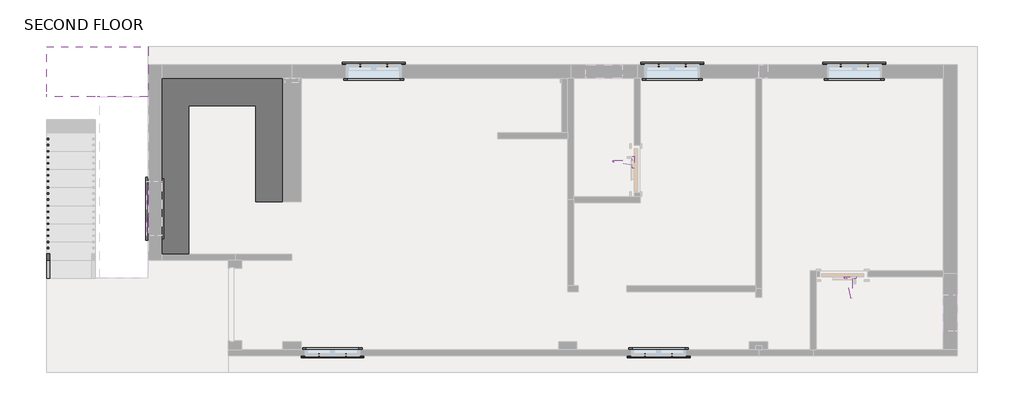
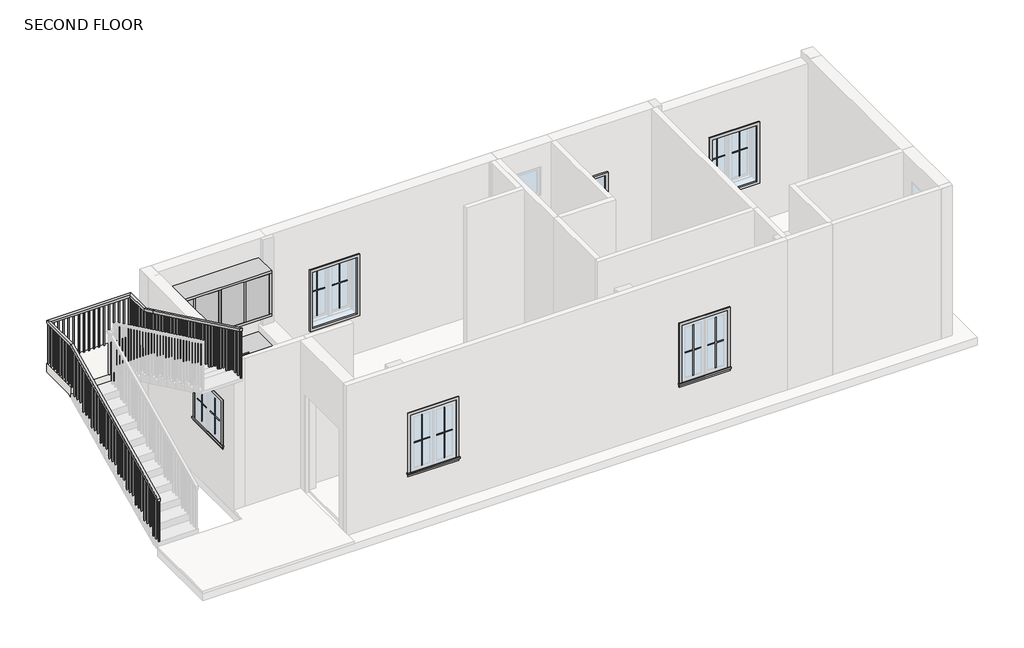
# One storey, part 3 of 3: 27 proxies, 1 railing, 1 slab.
"""IFC4 building model written with IfcOpenShell, lengths in millimetres."""

from ifc_helpers import new_model, si_unit, frame, origin, place, context, project, spatial, polyline, outline, extrude, faceted_brep, transform, mapped, element, save
from components import bel_door_closer_bel_door_closer_f210e2f3, bel_door_closer_bel_door_closer_a3520c2f, generic_models_3_generic_models_1_c5fb848b, muntin_pattern_2x2_muntin_pattern_2x2_1acec82f, muntin_pattern_2x2_muntin_pattern_2x2_43d02eee, muntin_pattern_2x2_muntin_pattern_2x2_d1c6e638, muntin_pattern_2x2_muntin_pattern_2x2_37b95fb2, trim_window_exterior_flat_with_sill_e4b28ec3, trim_window_exterior_flat_with_sill_84e24481, trim_window_interior_flat_picture_frame_39ff4276, trim_window_interior_flat_picture_frame_28d4e5dc

model = new_model("IFC4")

# Units and contexts
model_context = context("Model", 3, world=origin())
ifc_project = project(units=[si_unit("LENGTHUNIT", "METRE", prefix="MILLI")], contexts=[model_context])

# Site, building, storey
site = spatial("IfcSite", under=ifc_project)
building = spatial("IfcBuilding", under=site)
storey = spatial("IfcBuildingStorey", under=building, Name="SECOND FLOOR", Elevation=6400.8)

# Proxies
placement = place(None, origin())
bel_door_closer_bel_door_closer_shape = bel_door_closer_bel_door_closer_f210e2f3(model_context)
element("IfcBuildingElementProxy", 1, Name="BEL-Door Closer : BEL-Door Closer", ObjectType="BEL-Door Closer : BEL-Door Closer", at=placement, inside=storey, context=model_context, shape_type="MappedRepresentation", body=[
    mapped(bel_door_closer_bel_door_closer_shape, transform((6826.3533773, 1546.5642852, 8545.4957985), x_axis=(-1.0, 0.0, 0.0), y_axis=(0.0, 0.0, -1.0), z_axis=(0.0, -1.0, 0.0))),
])
bel_door_closer_bel_door_closer_2_shape = bel_door_closer_bel_door_closer_a3520c2f(model_context)
element("IfcBuildingElementProxy", 2, Name="BEL-Door Closer : BEL-Door Closer", ObjectType="BEL-Door Closer : BEL-Door Closer", at=placement, inside=storey, context=model_context, shape_type="MappedRepresentation", body=[
    mapped(bel_door_closer_bel_door_closer_2_shape, transform((3460.0408773, 3211.0767852, 8545.4957985), x_axis=(0.0, -1.0, 0.0), y_axis=(0.0, 0.0, 1.0), z_axis=(-1.0, 0.0, 0.0))),
])
generic_models_3_generic_models_1_shape = generic_models_3_generic_models_1_c5fb848b(model_context)
element("IfcBuildingElementProxy", 3, Name="Generic Models 3 : Generic Models 1", ObjectType="Generic Models 3 : Generic Models 1", at=placement, inside=storey, context=model_context, shape_type="MappedRepresentation", body=[
    mapped(generic_models_3_generic_models_1_shape, transform((0.0, 0.0, 0.0), x_axis=(1.0, 0.0, 0.0), y_axis=(0.0, 1.0, 0.0), z_axis=(0.0, 0.0, 1.0))),
])
muntin_pattern_2x2_muntin_pattern_2x2_shape = muntin_pattern_2x2_muntin_pattern_2x2_1acec82f(model_context)
element("IfcBuildingElementProxy", 4, Name="Muntin Pattern_2x2 : Muntin Pattern_2x2", ObjectType="Muntin Pattern_2x2 : Muntin Pattern_2x2", at=placement, inside=storey, context=model_context, shape_type="MappedRepresentation", body=[
    mapped(muntin_pattern_2x2_muntin_pattern_2x2_shape, transform((-1135.7716227, 5093.0392852, 7385.05), x_axis=(1.0, 0.0, 0.0), y_axis=(0.0, 1.0, 0.0), z_axis=(0.0, 0.0, 1.0))),
])
element("IfcBuildingElementProxy", 5, Name="Muntin Pattern_2x2 : Muntin Pattern_2x2", ObjectType="Muntin Pattern_2x2 : Muntin Pattern_2x2", at=placement, inside=storey, context=model_context, shape_type="MappedRepresentation", body=[
    mapped(muntin_pattern_2x2_muntin_pattern_2x2_shape, transform((3868.0283773, 5093.0392852, 7385.05), x_axis=(1.0, 0.0, 0.0), y_axis=(0.0, 1.0, 0.0), z_axis=(0.0, 0.0, 1.0))),
])
element("IfcBuildingElementProxy", 6, Name="Muntin Pattern_2x2 : Muntin Pattern_2x2", ObjectType="Muntin Pattern_2x2 : Muntin Pattern_2x2", at=placement, inside=storey, context=model_context, shape_type="MappedRepresentation", body=[
    mapped(muntin_pattern_2x2_muntin_pattern_2x2_shape, transform((6922.3783773, 5093.0392852, 7385.05), x_axis=(1.0, 0.0, 0.0), y_axis=(0.0, 1.0, 0.0), z_axis=(0.0, 0.0, 1.0))),
])
element("IfcBuildingElementProxy", 7, Name="Muntin Pattern_2x2 : Muntin Pattern_2x2", ObjectType="Muntin Pattern_2x2 : Muntin Pattern_2x2", at=placement, inside=storey, context=model_context, shape_type="MappedRepresentation", body=[
    mapped(muntin_pattern_2x2_muntin_pattern_2x2_shape, transform((4093.4533773, 235.2892852, 7385.05), x_axis=(-1.0, 0.0, 0.0), y_axis=(0.0, -1.0, 0.0), z_axis=(0.0, 0.0, 1.0))),
])
element("IfcBuildingElementProxy", 8, Name="Muntin Pattern_2x2 : Muntin Pattern_2x2", ObjectType="Muntin Pattern_2x2 : Muntin Pattern_2x2", at=placement, inside=storey, context=model_context, shape_type="MappedRepresentation", body=[
    mapped(muntin_pattern_2x2_muntin_pattern_2x2_shape, transform((-1373.8966227, 235.2892852, 7385.05), x_axis=(-1.0, 0.0, 0.0), y_axis=(0.0, -1.0, 0.0), z_axis=(0.0, 0.0, 1.0))),
])
muntin_pattern_2x2_muntin_pattern_2x2_2_shape = muntin_pattern_2x2_muntin_pattern_2x2_43d02eee(model_context)
element("IfcBuildingElementProxy", 9, Name="Muntin Pattern_2x2 : Muntin Pattern_2x2", ObjectType="Muntin Pattern_2x2 : Muntin Pattern_2x2", at=placement, inside=storey, context=model_context, shape_type="MappedRepresentation", body=[
    mapped(muntin_pattern_2x2_muntin_pattern_2x2_2_shape, transform((-681.7466227, 5093.0392852, 7385.05), x_axis=(-1.0, 0.0, 0.0), y_axis=(0.0, -1.0, 0.0), z_axis=(0.0, 0.0, 1.0))),
])
element("IfcBuildingElementProxy", 10, Name="Muntin Pattern_2x2 : Muntin Pattern_2x2", ObjectType="Muntin Pattern_2x2 : Muntin Pattern_2x2", at=placement, inside=storey, context=model_context, shape_type="MappedRepresentation", body=[
    mapped(muntin_pattern_2x2_muntin_pattern_2x2_2_shape, transform((4322.0533773, 5093.0392852, 7385.05), x_axis=(-1.0, 0.0, 0.0), y_axis=(0.0, -1.0, 0.0), z_axis=(0.0, 0.0, 1.0))),
])
element("IfcBuildingElementProxy", 11, Name="Muntin Pattern_2x2 : Muntin Pattern_2x2", ObjectType="Muntin Pattern_2x2 : Muntin Pattern_2x2", at=placement, inside=storey, context=model_context, shape_type="MappedRepresentation", body=[
    mapped(muntin_pattern_2x2_muntin_pattern_2x2_2_shape, transform((7376.4033773, 5093.0392852, 7385.05), x_axis=(-1.0, 0.0, 0.0), y_axis=(0.0, -1.0, 0.0), z_axis=(0.0, 0.0, 1.0))),
])
element("IfcBuildingElementProxy", 12, Name="Muntin Pattern_2x2 : Muntin Pattern_2x2", ObjectType="Muntin Pattern_2x2 : Muntin Pattern_2x2", at=placement, inside=storey, context=model_context, shape_type="MappedRepresentation", body=[
    mapped(muntin_pattern_2x2_muntin_pattern_2x2_2_shape, transform((3639.4283773, 235.2892852, 7385.05), x_axis=(1.0, 0.0, 0.0), y_axis=(0.0, 1.0, 0.0), z_axis=(0.0, 0.0, 1.0))),
])
element("IfcBuildingElementProxy", 13, Name="Muntin Pattern_2x2 : Muntin Pattern_2x2", ObjectType="Muntin Pattern_2x2 : Muntin Pattern_2x2", at=placement, inside=storey, context=model_context, shape_type="MappedRepresentation", body=[
    mapped(muntin_pattern_2x2_muntin_pattern_2x2_2_shape, transform((-1827.9216227, 235.2892852, 7385.05), x_axis=(1.0, 0.0, 0.0), y_axis=(0.0, 1.0, 0.0), z_axis=(0.0, 0.0, 1.0))),
])
muntin_pattern_2x2_muntin_pattern_2x2_3_shape = muntin_pattern_2x2_muntin_pattern_2x2_d1c6e638(model_context)
element("IfcBuildingElementProxy", 14, Name="Muntin Pattern_2x2 : Muntin Pattern_2x2", ObjectType="Muntin Pattern_2x2 : Muntin Pattern_2x2", at=placement, inside=storey, context=model_context, shape_type="MappedRepresentation", body=[
    mapped(muntin_pattern_2x2_muntin_pattern_2x2_3_shape, transform((-4683.8341227, 2462.5517852, 7689.85), x_axis=(0.0, 1.0, 0.0), y_axis=(-1.0, 0.0, 0.0), z_axis=(0.0, 0.0, 1.0))),
])
muntin_pattern_2x2_muntin_pattern_2x2_4_shape = muntin_pattern_2x2_muntin_pattern_2x2_37b95fb2(model_context)
element("IfcBuildingElementProxy", 15, Name="Muntin Pattern_2x2 : Muntin Pattern_2x2", ObjectType="Muntin Pattern_2x2 : Muntin Pattern_2x2", at=placement, inside=storey, context=model_context, shape_type="MappedRepresentation", body=[
    mapped(muntin_pattern_2x2_muntin_pattern_2x2_4_shape, transform((-4683.8341227, 2916.5767852, 7689.85), x_axis=(0.0, -1.0, 0.0), y_axis=(1.0, 0.0, 0.0), z_axis=(0.0, 0.0, 1.0))),
])
trim_window_exterior_flat_with_sill_shape = trim_window_exterior_flat_with_sill_e4b28ec3(model_context)
element("IfcBuildingElementProxy", 16, Name="Trim-Window-Exterior-Flat : with Sill", ObjectType="Trim-Window-Exterior-Flat : with Sill", at=placement, inside=storey, context=model_context, shape_type="MappedRepresentation", body=[
    mapped(trim_window_exterior_flat_with_sill_shape, transform((-908.7591227, 5102.5642852, 8534.4), x_axis=(-1.0, 0.0, 0.0), y_axis=(0.0, 0.0, 1.0), z_axis=(0.0, 1.0, 0.0))),
])
element("IfcBuildingElementProxy", 17, Name="Trim-Window-Exterior-Flat : with Sill", ObjectType="Trim-Window-Exterior-Flat : with Sill", at=placement, inside=storey, context=model_context, shape_type="MappedRepresentation", body=[
    mapped(trim_window_exterior_flat_with_sill_shape, transform((4095.0408773, 5102.5642852, 8534.4), x_axis=(-1.0, 0.0, 0.0), y_axis=(0.0, 0.0, 1.0), z_axis=(0.0, 1.0, 0.0))),
])
element("IfcBuildingElementProxy", 18, Name="Trim-Window-Exterior-Flat : with Sill", ObjectType="Trim-Window-Exterior-Flat : with Sill", at=placement, inside=storey, context=model_context, shape_type="MappedRepresentation", body=[
    mapped(trim_window_exterior_flat_with_sill_shape, transform((7149.3908773, 5102.5642852, 8534.4), x_axis=(-1.0, 0.0, 0.0), y_axis=(0.0, 0.0, 1.0), z_axis=(0.0, 1.0, 0.0))),
])
element("IfcBuildingElementProxy", 19, Name="Trim-Window-Exterior-Flat : with Sill", ObjectType="Trim-Window-Exterior-Flat : with Sill", at=placement, inside=storey, context=model_context, shape_type="MappedRepresentation", body=[
    mapped(trim_window_exterior_flat_with_sill_shape, transform((3866.4408773, 225.7642852, 8534.4), x_axis=(1.0, 0.0, 0.0), y_axis=(0.0, 0.0, 1.0), z_axis=(0.0, -1.0, 0.0))),
])
element("IfcBuildingElementProxy", 20, Name="Trim-Window-Exterior-Flat : with Sill", ObjectType="Trim-Window-Exterior-Flat : with Sill", at=placement, inside=storey, context=model_context, shape_type="MappedRepresentation", body=[
    mapped(trim_window_exterior_flat_with_sill_shape, transform((-1600.9091227, 225.7642852, 8534.4), x_axis=(1.0, 0.0, 0.0), y_axis=(0.0, 0.0, 1.0), z_axis=(0.0, -1.0, 0.0))),
])
trim_window_exterior_flat_with_sill_2_shape = trim_window_exterior_flat_with_sill_84e24481(model_context)
element("IfcBuildingElementProxy", 21, Name="Trim-Window-Exterior-Flat : with Sill", ObjectType="Trim-Window-Exterior-Flat : with Sill", at=placement, inside=storey, context=model_context, shape_type="MappedRepresentation", body=[
    mapped(trim_window_exterior_flat_with_sill_2_shape, transform((-4693.3591227, 2689.5642852, 8534.4), x_axis=(0.0, -1.0, 0.0), y_axis=(0.0, 0.0, 1.0), z_axis=(-1.0, 0.0, 0.0))),
])
trim_window_interior_flat_picture_frame_shape = trim_window_interior_flat_picture_frame_39ff4276(model_context)
element("IfcBuildingElementProxy", 22, Name="Trim-Window-Interior-Flat : Picture Frame", ObjectType="Trim-Window-Interior-Flat : Picture Frame", at=placement, inside=storey, context=model_context, shape_type="MappedRepresentation", body=[
    mapped(trim_window_interior_flat_picture_frame_shape, transform((-908.7591227, 4873.9642852, 8534.4), x_axis=(1.0, 0.0, 0.0), y_axis=(0.0, 0.0, 1.0), z_axis=(0.0, -1.0, 0.0))),
])
element("IfcBuildingElementProxy", 23, Name="Trim-Window-Interior-Flat : Picture Frame", ObjectType="Trim-Window-Interior-Flat : Picture Frame", at=placement, inside=storey, context=model_context, shape_type="MappedRepresentation", body=[
    mapped(trim_window_interior_flat_picture_frame_shape, transform((4095.0408773, 4873.9642852, 8534.4), x_axis=(1.0, 0.0, 0.0), y_axis=(0.0, 0.0, 1.0), z_axis=(0.0, -1.0, 0.0))),
])
element("IfcBuildingElementProxy", 24, Name="Trim-Window-Interior-Flat : Picture Frame", ObjectType="Trim-Window-Interior-Flat : Picture Frame", at=placement, inside=storey, context=model_context, shape_type="MappedRepresentation", body=[
    mapped(trim_window_interior_flat_picture_frame_shape, transform((7149.3908773, 4873.9642852, 8534.4), x_axis=(1.0, 0.0, 0.0), y_axis=(0.0, 0.0, 1.0), z_axis=(0.0, -1.0, 0.0))),
])
element("IfcBuildingElementProxy", 25, Name="Trim-Window-Interior-Flat : Picture Frame", ObjectType="Trim-Window-Interior-Flat : Picture Frame", at=placement, inside=storey, context=model_context, shape_type="MappedRepresentation", body=[
    mapped(trim_window_interior_flat_picture_frame_shape, transform((3866.4408773, 327.3642852, 8534.4), x_axis=(-1.0, 0.0, 0.0), y_axis=(0.0, 0.0, 1.0), z_axis=(0.0, 1.0, 0.0))),
])
element("IfcBuildingElementProxy", 26, Name="Trim-Window-Interior-Flat : Picture Frame", ObjectType="Trim-Window-Interior-Flat : Picture Frame", at=placement, inside=storey, context=model_context, shape_type="MappedRepresentation", body=[
    mapped(trim_window_interior_flat_picture_frame_shape, transform((-1600.9091227, 327.3642852, 8534.4), x_axis=(-1.0, 0.0, 0.0), y_axis=(0.0, 0.0, 1.0), z_axis=(0.0, 1.0, 0.0))),
])
trim_window_interior_flat_picture_frame_2_shape = trim_window_interior_flat_picture_frame_28d4e5dc(model_context)
element("IfcBuildingElementProxy", 27, Name="Trim-Window-Interior-Flat : Picture Frame", ObjectType="Trim-Window-Interior-Flat : Picture Frame", at=placement, inside=storey, context=model_context, shape_type="MappedRepresentation", body=[
    mapped(trim_window_interior_flat_picture_frame_2_shape, transform((-4464.7591227, 2689.5642852, 8534.4), x_axis=(0.0, 1.0, 0.0), y_axis=(0.0, 0.0, 1.0), z_axis=(1.0, 0.0, 0.0))),
])

# Railing
element("IfcRailing", 28, ObjectType="Handrail - Rectangular", at=placement, inside=storey, context=model_context, shape_type="SolidModel", body=[
    faceted_brep([(-6395.1591227, 1521.1642852, 7460.6727273), (-6395.1591227, 1521.1642852, 7404.3834559), (-6344.3591227, 1521.1642852, 7404.3834559), (-6344.3591227, 1521.1642852, 7460.6727273), (-6395.1591227, 4569.1642852, 8915.4), (-6395.1591227, 4580.6656156, 8864.6), (-6344.3591227, 4580.6656156, 8864.6), (-6344.3591227, 4569.1642852, 8915.4), (-6395.1591227, 5407.3642852, 8915.4), (-6395.1591227, 5407.3642852, 8864.6), (-6344.3591227, 5356.5642852, 8864.6), (-6344.3591227, 5356.5642852, 8915.4), (-4693.3591227, 5407.3642852, 8915.4), (-4693.3591227, 5407.3642852, 8864.6), (-4744.1591227, 5356.5642852, 8864.6), (-4744.1591227, 5356.5642852, 8915.4), (-4693.3591227, 4873.9642852, 8915.4), (-4693.3591227, 4862.4629548, 8864.6), (-4744.1591227, 4862.4629548, 8864.6), (-4744.1591227, 4873.9642852, 8915.4), (-4693.3591227, 4569.1642852, 9060.8727273), (-4693.3591227, 4547.2832222, 9015.0266906), (-4744.1591227, 4547.2832222, 9015.0266906), (-4744.1591227, 4569.1642852, 9060.8727273), (-4693.3591227, 1521.1642852, 10515.6), (-4744.1591227, 1521.1642852, 10515.6), (-4744.1591227, 1521.1642852, 10459.3107287), (-4693.3591227, 1521.1642852, 10459.3107287)], [[[0, 1, 2, 3]], [[1, 0, 4, 5]], [[2, 1, 5, 6]], [[3, 2, 6, 7]], [[0, 3, 7, 4]], [[5, 4, 8, 9]], [[6, 5, 9, 10]], [[7, 6, 10, 11]], [[4, 7, 11, 8]], [[9, 8, 12, 13]], [[10, 9, 13, 14]], [[11, 10, 14, 15]], [[8, 11, 15, 12]], [[13, 12, 16, 17]], [[14, 13, 17, 18]], [[15, 14, 18, 19]], [[12, 15, 19, 16]], [[17, 16, 20, 21]], [[18, 17, 21, 22]], [[19, 18, 22, 23]], [[16, 19, 23, 20]], [[24, 25, 26, 27]], [[21, 20, 24, 27]], [[22, 21, 27, 26]], [[23, 22, 26, 25]], [[20, 23, 25, 24]]]),
    extrude(outline(polyline([(1632.2892852, 10406.2737969), (1632.2892852, 9455.7272727), (1613.2392852, 9455.7272727), (1613.2392852, 10415.3658423), (1632.2892852, 10406.2737969)])), frame((-4728.2841227, 0.0, 0.0), z_axis=(1.0, 0.0, 0.0), x_axis=(0.0, 1.0, 0.0)), (0.0, 0.0, 1.0), 19.05),
    extrude(outline(polyline([(1733.8892852, 10357.7828878), (1733.8892852, 9455.7272727), (1714.8392852, 9455.7272727), (1714.8392852, 10366.8749332), (1733.8892852, 10357.7828878)])), frame((-4728.2841227, 0.0, 0.0), z_axis=(1.0, 0.0, 0.0), x_axis=(0.0, 1.0, 0.0)), (0.0, 0.0, 1.0), 19.05),
    extrude(outline(polyline([(1835.4892852, 10309.2919787), (1835.4892852, 9455.7272727), (1816.4392852, 9455.7272727), (1816.4392852, 10318.3840241), (1835.4892852, 10309.2919787)])), frame((-4728.2841227, 0.0, 0.0), z_axis=(1.0, 0.0, 0.0), x_axis=(0.0, 1.0, 0.0)), (0.0, 0.0, 1.0), 19.05),
    extrude(outline(polyline([(1937.0892852, 10260.8010696), (1937.0892852, 9310.2545455), (1918.0392852, 9310.2545455), (1918.0392852, 10269.893115), (1937.0892852, 10260.8010696)])), frame((-4728.2841227, 0.0, 0.0), z_axis=(1.0, 0.0, 0.0), x_axis=(0.0, 1.0, 0.0)), (0.0, 0.0, 1.0), 19.05),
    extrude(outline(polyline([(2038.6892852, 10212.3101605), (2038.6892852, 9310.2545455), (2019.6392852, 9310.2545455), (2019.6392852, 10221.4022059), (2038.6892852, 10212.3101605)])), frame((-4728.2841227, 0.0, 0.0), z_axis=(1.0, 0.0, 0.0), x_axis=(0.0, 1.0, 0.0)), (0.0, 0.0, 1.0), 19.05),
    extrude(outline(polyline([(2140.2892852, 10163.8192514), (2140.2892852, 9310.2545455), (2121.2392852, 9310.2545455), (2121.2392852, 10172.9112969), (2140.2892852, 10163.8192514)])), frame((-4728.2841227, 0.0, 0.0), z_axis=(1.0, 0.0, 0.0), x_axis=(0.0, 1.0, 0.0)), (0.0, 0.0, 1.0), 19.05),
    extrude(outline(polyline([(2241.8892852, 10115.3283423), (2241.8892852, 9164.7818182), (2222.8392852, 9164.7818182), (2222.8392852, 10124.4203878), (2241.8892852, 10115.3283423)])), frame((-4728.2841227, 0.0, 0.0), z_axis=(1.0, 0.0, 0.0), x_axis=(0.0, 1.0, 0.0)), (0.0, 0.0, 1.0), 19.05),
    extrude(outline(polyline([(2343.4892852, 10066.8374332), (2343.4892852, 9164.7818182), (2324.4392852, 9164.7818182), (2324.4392852, 10075.9294787), (2343.4892852, 10066.8374332)])), frame((-4728.2841227, 0.0, 0.0), z_axis=(1.0, 0.0, 0.0), x_axis=(0.0, 1.0, 0.0)), (0.0, 0.0, 1.0), 19.05),
    extrude(outline(polyline([(2445.0892852, 10018.3465241), (2445.0892852, 9164.7818182), (2426.0392852, 9164.7818182), (2426.0392852, 10027.4385696), (2445.0892852, 10018.3465241)])), frame((-4728.2841227, 0.0, 0.0), z_axis=(1.0, 0.0, 0.0), x_axis=(0.0, 1.0, 0.0)), (0.0, 0.0, 1.0), 19.05),
    extrude(outline(polyline([(2546.6892852, 9969.855615), (2546.6892852, 9019.3090909), (2527.6392852, 9019.3090909), (2527.6392852, 9978.9476605), (2546.6892852, 9969.855615)])), frame((-4728.2841227, 0.0, 0.0), z_axis=(1.0, 0.0, 0.0), x_axis=(0.0, 1.0, 0.0)), (0.0, 0.0, 1.0), 19.05),
    extrude(outline(polyline([(2648.2892852, 9921.3647059), (2648.2892852, 9019.3090909), (2629.2392852, 9019.3090909), (2629.2392852, 9930.4567514), (2648.2892852, 9921.3647059)])), frame((-4728.2841227, 0.0, 0.0), z_axis=(1.0, 0.0, 0.0), x_axis=(0.0, 1.0, 0.0)), (0.0, 0.0, 1.0), 19.05),
    extrude(outline(polyline([(2749.8892852, 9872.8737969), (2749.8892852, 9019.3090909), (2730.8392852, 9019.3090909), (2730.8392852, 9881.9658423), (2749.8892852, 9872.8737969)])), frame((-4728.2841227, 0.0, 0.0), z_axis=(1.0, 0.0, 0.0), x_axis=(0.0, 1.0, 0.0)), (0.0, 0.0, 1.0), 19.05),
    extrude(outline(polyline([(2851.4892852, 9824.3828878), (2851.4892852, 8873.8363636), (2832.4392852, 8873.8363636), (2832.4392852, 9833.4749332), (2851.4892852, 9824.3828878)])), frame((-4728.2841227, 0.0, 0.0), z_axis=(1.0, 0.0, 0.0), x_axis=(0.0, 1.0, 0.0)), (0.0, 0.0, 1.0), 19.05),
    extrude(outline(polyline([(2953.0892852, 9775.8919787), (2953.0892852, 8873.8363636), (2934.0392852, 8873.8363636), (2934.0392852, 9784.9840241), (2953.0892852, 9775.8919787)])), frame((-4728.2841227, 0.0, 0.0), z_axis=(1.0, 0.0, 0.0), x_axis=(0.0, 1.0, 0.0)), (0.0, 0.0, 1.0), 19.05),
    extrude(outline(polyline([(3054.6892852, 9727.4010696), (3054.6892852, 8873.8363636), (3035.6392852, 8873.8363636), (3035.6392852, 9736.493115), (3054.6892852, 9727.4010696)])), frame((-4728.2841227, 0.0, 0.0), z_axis=(1.0, 0.0, 0.0), x_axis=(0.0, 1.0, 0.0)), (0.0, 0.0, 1.0), 19.05),
    extrude(outline(polyline([(3156.2892852, 9678.9101605), (3156.2892852, 8728.3636364), (3137.2392852, 8728.3636364), (3137.2392852, 9688.0022059), (3156.2892852, 9678.9101605)])), frame((-4728.2841227, 0.0, 0.0), z_axis=(1.0, 0.0, 0.0), x_axis=(0.0, 1.0, 0.0)), (0.0, 0.0, 1.0), 19.05),
    extrude(outline(polyline([(3257.8892852, 9630.4192514), (3257.8892852, 8728.3636364), (3238.8392852, 8728.3636364), (3238.8392852, 9639.5112969), (3257.8892852, 9630.4192514)])), frame((-4728.2841227, 0.0, 0.0), z_axis=(1.0, 0.0, 0.0), x_axis=(0.0, 1.0, 0.0)), (0.0, 0.0, 1.0), 19.05),
    extrude(outline(polyline([(3359.4892852, 9581.9283423), (3359.4892852, 8728.3636364), (3340.4392852, 8728.3636364), (3340.4392852, 9591.0203878), (3359.4892852, 9581.9283423)])), frame((-4728.2841227, 0.0, 0.0), z_axis=(1.0, 0.0, 0.0), x_axis=(0.0, 1.0, 0.0)), (0.0, 0.0, 1.0), 19.05),
    extrude(outline(polyline([(3461.0892852, 9533.4374332), (3461.0892852, 8582.8909091), (3442.0392852, 8582.8909091), (3442.0392852, 9542.5294787), (3461.0892852, 9533.4374332)])), frame((-4728.2841227, 0.0, 0.0), z_axis=(1.0, 0.0, 0.0), x_axis=(0.0, 1.0, 0.0)), (0.0, 0.0, 1.0), 19.05),
    extrude(outline(polyline([(3562.6892852, 9484.9465241), (3562.6892852, 8582.8909091), (3543.6392852, 8582.8909091), (3543.6392852, 9494.0385696), (3562.6892852, 9484.9465241)])), frame((-4728.2841227, 0.0, 0.0), z_axis=(1.0, 0.0, 0.0), x_axis=(0.0, 1.0, 0.0)), (0.0, 0.0, 1.0), 19.05),
    extrude(outline(polyline([(3664.2892852, 9436.455615), (3664.2892852, 8582.8909091), (3645.2392852, 8582.8909091), (3645.2392852, 9445.5476605), (3664.2892852, 9436.455615)])), frame((-4728.2841227, 0.0, 0.0), z_axis=(1.0, 0.0, 0.0), x_axis=(0.0, 1.0, 0.0)), (0.0, 0.0, 1.0), 19.05),
    extrude(outline(polyline([(3765.8892852, 9387.9647059), (3765.8892852, 8437.4181818), (3746.8392852, 8437.4181818), (3746.8392852, 9397.0567514), (3765.8892852, 9387.9647059)])), frame((-4728.2841227, 0.0, 0.0), z_axis=(1.0, 0.0, 0.0), x_axis=(0.0, 1.0, 0.0)), (0.0, 0.0, 1.0), 19.05),
    extrude(outline(polyline([(3867.4892852, 9339.4737969), (3867.4892852, 8437.4181818), (3848.4392852, 8437.4181818), (3848.4392852, 9348.5658423), (3867.4892852, 9339.4737969)])), frame((-4728.2841227, 0.0, 0.0), z_axis=(1.0, 0.0, 0.0), x_axis=(0.0, 1.0, 0.0)), (0.0, 0.0, 1.0), 19.05),
    extrude(outline(polyline([(3969.0892852, 9290.9828878), (3969.0892852, 8437.4181818), (3950.0392852, 8437.4181818), (3950.0392852, 9300.0749332), (3969.0892852, 9290.9828878)])), frame((-4728.2841227, 0.0, 0.0), z_axis=(1.0, 0.0, 0.0), x_axis=(0.0, 1.0, 0.0)), (0.0, 0.0, 1.0), 19.05),
    extrude(outline(polyline([(4070.6892852, 9242.4919787), (4070.6892852, 8291.9454545), (4051.6392852, 8291.9454545), (4051.6392852, 9251.5840241), (4070.6892852, 9242.4919787)])), frame((-4728.2841227, 0.0, 0.0), z_axis=(1.0, 0.0, 0.0), x_axis=(0.0, 1.0, 0.0)), (0.0, 0.0, 1.0), 19.05),
    extrude(outline(polyline([(4172.2892852, 9194.0010696), (4172.2892852, 8291.9454545), (4153.2392852, 8291.9454545), (4153.2392852, 9203.093115), (4172.2892852, 9194.0010696)])), frame((-4728.2841227, 0.0, 0.0), z_axis=(1.0, 0.0, 0.0), x_axis=(0.0, 1.0, 0.0)), (0.0, 0.0, 1.0), 19.05),
    extrude(outline(polyline([(4273.8892852, 9145.5101605), (4273.8892852, 8291.9454545), (4254.8392852, 8291.9454545), (4254.8392852, 9154.6022059), (4273.8892852, 9145.5101605)])), frame((-4728.2841227, 0.0, 0.0), z_axis=(1.0, 0.0, 0.0), x_axis=(0.0, 1.0, 0.0)), (0.0, 0.0, 1.0), 19.05),
    extrude(outline(polyline([(4375.4892852, 9097.0192514), (4375.4892852, 8146.4727273), (4356.4392852, 8146.4727273), (4356.4392852, 9106.1112969), (4375.4892852, 9097.0192514)])), frame((-4728.2841227, 0.0, 0.0), z_axis=(1.0, 0.0, 0.0), x_axis=(0.0, 1.0, 0.0)), (0.0, 0.0, 1.0), 19.05),
    extrude(outline(polyline([(4477.0892852, 9048.5283423), (4477.0892852, 8146.4727273), (4458.0392852, 8146.4727273), (4458.0392852, 9057.6203878), (4477.0892852, 9048.5283423)])), frame((-4728.2841227, 0.0, 0.0), z_axis=(1.0, 0.0, 0.0), x_axis=(0.0, 1.0, 0.0)), (0.0, 0.0, 1.0), 19.05),
    extrude(outline(polyline([(4680.2892852, 8951.5465241), (4680.2892852, 8001.0), (4661.2392852, 8001.0), (4661.2392852, 8960.6385696), (4680.2892852, 8951.5465241)])), frame((-4728.2841227, 0.0, 0.0), z_axis=(1.0, 0.0, 0.0), x_axis=(0.0, 1.0, 0.0)), (0.0, 0.0, 1.0), 19.05),
    extrude(outline(polyline([(4781.8892852, 8903.055615), (4781.8892852, 8001.0), (4762.8392852, 8001.0), (4762.8392852, 8912.1476605), (4781.8892852, 8903.055615)])), frame((-4728.2841227, 0.0, 0.0), z_axis=(1.0, 0.0, 0.0), x_axis=(0.0, 1.0, 0.0)), (0.0, 0.0, 1.0), 19.05),
    extrude(outline(polyline([(-4709.2341227, 4883.4892852), (-4709.2341227, 4864.4392852), (-4728.2841227, 4864.4392852), (-4728.2841227, 4883.4892852), (-4709.2341227, 4883.4892852)])), frame((0.0, 0.0, 8001.0), z_axis=(0.0, 0.0, 1.0), x_axis=(1.0, 0.0, 0.0)), (0.0, 0.0, 1.0), 863.6),
    extrude(outline(polyline([(-4709.2341227, 4985.0892852), (-4709.2341227, 4966.0392852), (-4728.2841227, 4966.0392852), (-4728.2841227, 4985.0892852), (-4709.2341227, 4985.0892852)])), frame((0.0, 0.0, 8001.0), z_axis=(0.0, 0.0, 1.0), x_axis=(1.0, 0.0, 0.0)), (0.0, 0.0, 1.0), 863.6),
    extrude(outline(polyline([(-4709.2341227, 5086.6892852), (-4709.2341227, 5067.6392852), (-4728.2841227, 5067.6392852), (-4728.2841227, 5086.6892852), (-4709.2341227, 5086.6892852)])), frame((0.0, 0.0, 8001.0), z_axis=(0.0, 0.0, 1.0), x_axis=(1.0, 0.0, 0.0)), (0.0, 0.0, 1.0), 863.6),
    extrude(outline(polyline([(-4709.2341227, 5188.2892852), (-4709.2341227, 5169.2392852), (-4728.2841227, 5169.2392852), (-4728.2841227, 5188.2892852), (-4709.2341227, 5188.2892852)])), frame((0.0, 0.0, 8001.0), z_axis=(0.0, 0.0, 1.0), x_axis=(1.0, 0.0, 0.0)), (0.0, 0.0, 1.0), 863.6),
    extrude(outline(polyline([(-4709.2341227, 5289.8892852), (-4709.2341227, 5270.8392852), (-4728.2841227, 5270.8392852), (-4728.2841227, 5289.8892852), (-4709.2341227, 5289.8892852)])), frame((0.0, 0.0, 8001.0), z_axis=(0.0, 0.0, 1.0), x_axis=(1.0, 0.0, 0.0)), (0.0, 0.0, 1.0), 863.6),
    extrude(outline(polyline([(-4753.6841227, 5391.4892852), (-4734.6341227, 5391.4892852), (-4734.6341227, 5372.4392852), (-4753.6841227, 5372.4392852), (-4753.6841227, 5391.4892852)])), frame((0.0, 0.0, 8001.0), z_axis=(0.0, 0.0, 1.0), x_axis=(1.0, 0.0, 0.0)), (0.0, 0.0, 1.0), 863.6),
    extrude(outline(polyline([(-4855.2841227, 5391.4892852), (-4836.2341227, 5391.4892852), (-4836.2341227, 5372.4392852), (-4855.2841227, 5372.4392852), (-4855.2841227, 5391.4892852)])), frame((0.0, 0.0, 8001.0), z_axis=(0.0, 0.0, 1.0), x_axis=(1.0, 0.0, 0.0)), (0.0, 0.0, 1.0), 863.6),
    extrude(outline(polyline([(-4956.8841227, 5391.4892852), (-4937.8341227, 5391.4892852), (-4937.8341227, 5372.4392852), (-4956.8841227, 5372.4392852), (-4956.8841227, 5391.4892852)])), frame((0.0, 0.0, 8001.0), z_axis=(0.0, 0.0, 1.0), x_axis=(1.0, 0.0, 0.0)), (0.0, 0.0, 1.0), 863.6),
    extrude(outline(polyline([(-5058.4841227, 5391.4892852), (-5039.4341227, 5391.4892852), (-5039.4341227, 5372.4392852), (-5058.4841227, 5372.4392852), (-5058.4841227, 5391.4892852)])), frame((0.0, 0.0, 8001.0), z_axis=(0.0, 0.0, 1.0), x_axis=(1.0, 0.0, 0.0)), (0.0, 0.0, 1.0), 863.6),
    extrude(outline(polyline([(-5160.0841227, 5391.4892852), (-5141.0341227, 5391.4892852), (-5141.0341227, 5372.4392852), (-5160.0841227, 5372.4392852), (-5160.0841227, 5391.4892852)])), frame((0.0, 0.0, 8001.0), z_axis=(0.0, 0.0, 1.0), x_axis=(1.0, 0.0, 0.0)), (0.0, 0.0, 1.0), 863.6),
    extrude(outline(polyline([(-5261.6841227, 5391.4892852), (-5242.6341227, 5391.4892852), (-5242.6341227, 5372.4392852), (-5261.6841227, 5372.4392852), (-5261.6841227, 5391.4892852)])), frame((0.0, 0.0, 8001.0), z_axis=(0.0, 0.0, 1.0), x_axis=(1.0, 0.0, 0.0)), (0.0, 0.0, 1.0), 863.6),
    extrude(outline(polyline([(-5363.2841227, 5391.4892852), (-5344.2341227, 5391.4892852), (-5344.2341227, 5372.4392852), (-5363.2841227, 5372.4392852), (-5363.2841227, 5391.4892852)])), frame((0.0, 0.0, 8001.0), z_axis=(0.0, 0.0, 1.0), x_axis=(1.0, 0.0, 0.0)), (0.0, 0.0, 1.0), 863.6),
    extrude(outline(polyline([(-5464.8841227, 5391.4892852), (-5445.8341227, 5391.4892852), (-5445.8341227, 5372.4392852), (-5464.8841227, 5372.4392852), (-5464.8841227, 5391.4892852)])), frame((0.0, 0.0, 8001.0), z_axis=(0.0, 0.0, 1.0), x_axis=(1.0, 0.0, 0.0)), (0.0, 0.0, 1.0), 863.6),
    extrude(outline(polyline([(-5566.4841227, 5391.4892852), (-5547.4341227, 5391.4892852), (-5547.4341227, 5372.4392852), (-5566.4841227, 5372.4392852), (-5566.4841227, 5391.4892852)])), frame((0.0, 0.0, 8001.0), z_axis=(0.0, 0.0, 1.0), x_axis=(1.0, 0.0, 0.0)), (0.0, 0.0, 1.0), 863.6),
    extrude(outline(polyline([(-5668.0841227, 5391.4892852), (-5649.0341227, 5391.4892852), (-5649.0341227, 5372.4392852), (-5668.0841227, 5372.4392852), (-5668.0841227, 5391.4892852)])), frame((0.0, 0.0, 8001.0), z_axis=(0.0, 0.0, 1.0), x_axis=(1.0, 0.0, 0.0)), (0.0, 0.0, 1.0), 863.6),
    extrude(outline(polyline([(-5769.6841227, 5391.4892852), (-5750.6341227, 5391.4892852), (-5750.6341227, 5372.4392852), (-5769.6841227, 5372.4392852), (-5769.6841227, 5391.4892852)])), frame((0.0, 0.0, 8001.0), z_axis=(0.0, 0.0, 1.0), x_axis=(1.0, 0.0, 0.0)), (0.0, 0.0, 1.0), 863.6),
    extrude(outline(polyline([(-5871.2841227, 5391.4892852), (-5852.2341227, 5391.4892852), (-5852.2341227, 5372.4392852), (-5871.2841227, 5372.4392852), (-5871.2841227, 5391.4892852)])), frame((0.0, 0.0, 8001.0), z_axis=(0.0, 0.0, 1.0), x_axis=(1.0, 0.0, 0.0)), (0.0, 0.0, 1.0), 863.6),
    extrude(outline(polyline([(-5972.8841227, 5391.4892852), (-5953.8341227, 5391.4892852), (-5953.8341227, 5372.4392852), (-5972.8841227, 5372.4392852), (-5972.8841227, 5391.4892852)])), frame((0.0, 0.0, 8001.0), z_axis=(0.0, 0.0, 1.0), x_axis=(1.0, 0.0, 0.0)), (0.0, 0.0, 1.0), 863.6),
    extrude(outline(polyline([(-6074.4841227, 5391.4892852), (-6055.4341227, 5391.4892852), (-6055.4341227, 5372.4392852), (-6074.4841227, 5372.4392852), (-6074.4841227, 5391.4892852)])), frame((0.0, 0.0, 8001.0), z_axis=(0.0, 0.0, 1.0), x_axis=(1.0, 0.0, 0.0)), (0.0, 0.0, 1.0), 863.6),
    extrude(outline(polyline([(-6176.0841227, 5391.4892852), (-6157.0341227, 5391.4892852), (-6157.0341227, 5372.4392852), (-6176.0841227, 5372.4392852), (-6176.0841227, 5391.4892852)])), frame((0.0, 0.0, 8001.0), z_axis=(0.0, 0.0, 1.0), x_axis=(1.0, 0.0, 0.0)), (0.0, 0.0, 1.0), 863.6),
    extrude(outline(polyline([(-6277.6841227, 5391.4892852), (-6258.6341227, 5391.4892852), (-6258.6341227, 5372.4392852), (-6277.6841227, 5372.4392852), (-6277.6841227, 5391.4892852)])), frame((0.0, 0.0, 8001.0), z_axis=(0.0, 0.0, 1.0), x_axis=(1.0, 0.0, 0.0)), (0.0, 0.0, 1.0), 863.6),
    extrude(outline(polyline([(-6379.2841227, 5270.8392852), (-6379.2841227, 5289.8892852), (-6360.2341227, 5289.8892852), (-6360.2341227, 5270.8392852), (-6379.2841227, 5270.8392852)])), frame((0.0, 0.0, 8001.0), z_axis=(0.0, 0.0, 1.0), x_axis=(1.0, 0.0, 0.0)), (0.0, 0.0, 1.0), 863.6),
    extrude(outline(polyline([(-6379.2841227, 5169.2392852), (-6379.2841227, 5188.2892852), (-6360.2341227, 5188.2892852), (-6360.2341227, 5169.2392852), (-6379.2841227, 5169.2392852)])), frame((0.0, 0.0, 8001.0), z_axis=(0.0, 0.0, 1.0), x_axis=(1.0, 0.0, 0.0)), (0.0, 0.0, 1.0), 863.6),
    extrude(outline(polyline([(-6379.2841227, 5067.6392852), (-6379.2841227, 5086.6892852), (-6360.2341227, 5086.6892852), (-6360.2341227, 5067.6392852), (-6379.2841227, 5067.6392852)])), frame((0.0, 0.0, 8001.0), z_axis=(0.0, 0.0, 1.0), x_axis=(1.0, 0.0, 0.0)), (0.0, 0.0, 1.0), 863.6),
    extrude(outline(polyline([(-6379.2841227, 4966.0392852), (-6379.2841227, 4985.0892852), (-6360.2341227, 4985.0892852), (-6360.2341227, 4966.0392852), (-6379.2841227, 4966.0392852)])), frame((0.0, 0.0, 8001.0), z_axis=(0.0, 0.0, 1.0), x_axis=(1.0, 0.0, 0.0)), (0.0, 0.0, 1.0), 863.6),
    extrude(outline(polyline([(-6379.2841227, 4864.4392852), (-6379.2841227, 4883.4892852), (-6360.2341227, 4883.4892852), (-6360.2341227, 4864.4392852), (-6379.2841227, 4864.4392852)])), frame((0.0, 0.0, 8001.0), z_axis=(0.0, 0.0, 1.0), x_axis=(1.0, 0.0, 0.0)), (0.0, 0.0, 1.0), 863.6),
    extrude(outline(polyline([(-6379.2841227, 4762.8392852), (-6379.2841227, 4781.8892852), (-6360.2341227, 4781.8892852), (-6360.2341227, 4762.8392852), (-6379.2841227, 4762.8392852)])), frame((0.0, 0.0, 8001.0), z_axis=(0.0, 0.0, 1.0), x_axis=(1.0, 0.0, 0.0)), (0.0, 0.0, 1.0), 863.6),
    extrude(outline(polyline([(-6379.2841227, 4661.2392852), (-6379.2841227, 4680.2892852), (-6360.2341227, 4680.2892852), (-6360.2341227, 4661.2392852), (-6379.2841227, 4661.2392852)])), frame((0.0, 0.0, 8001.0), z_axis=(0.0, 0.0, 1.0), x_axis=(1.0, 0.0, 0.0)), (0.0, 0.0, 1.0), 863.6),
    extrude(outline(polyline([(4477.0892852, 8815.1658423), (4477.0892852, 7855.5272727), (4458.0392852, 7855.5272727), (4458.0392852, 8806.0737969), (4477.0892852, 8815.1658423)])), frame((-6379.2841227, 0.0, 0.0), z_axis=(1.0, 0.0, 0.0), x_axis=(0.0, 1.0, 0.0)), (0.0, 0.0, 1.0), 19.05),
    extrude(outline(polyline([(4375.4892852, 8766.6749332), (4375.4892852, 7855.5272727), (4356.4392852, 7855.5272727), (4356.4392852, 8757.5828878), (4375.4892852, 8766.6749332)])), frame((-6379.2841227, 0.0, 0.0), z_axis=(1.0, 0.0, 0.0), x_axis=(0.0, 1.0, 0.0)), (0.0, 0.0, 1.0), 19.05),
    extrude(outline(polyline([(4273.8892852, 8718.1840241), (4273.8892852, 7855.5272727), (4254.8392852, 7855.5272727), (4254.8392852, 8709.0919787), (4273.8892852, 8718.1840241)])), frame((-6379.2841227, 0.0, 0.0), z_axis=(1.0, 0.0, 0.0), x_axis=(0.0, 1.0, 0.0)), (0.0, 0.0, 1.0), 19.05),
    extrude(outline(polyline([(4172.2892852, 8669.693115), (4172.2892852, 7710.0545455), (4153.2392852, 7710.0545455), (4153.2392852, 8660.6010696), (4172.2892852, 8669.693115)])), frame((-6379.2841227, 0.0, 0.0), z_axis=(1.0, 0.0, 0.0), x_axis=(0.0, 1.0, 0.0)), (0.0, 0.0, 1.0), 19.05),
    extrude(outline(polyline([(4070.6892852, 8621.2022059), (4070.6892852, 7710.0545455), (4051.6392852, 7710.0545455), (4051.6392852, 8612.1101605), (4070.6892852, 8621.2022059)])), frame((-6379.2841227, 0.0, 0.0), z_axis=(1.0, 0.0, 0.0), x_axis=(0.0, 1.0, 0.0)), (0.0, 0.0, 1.0), 19.05),
    extrude(outline(polyline([(3969.0892852, 8572.7112969), (3969.0892852, 7710.0545455), (3950.0392852, 7710.0545455), (3950.0392852, 8563.6192514), (3969.0892852, 8572.7112969)])), frame((-6379.2841227, 0.0, 0.0), z_axis=(1.0, 0.0, 0.0), x_axis=(0.0, 1.0, 0.0)), (0.0, 0.0, 1.0), 19.05),
    extrude(outline(polyline([(3867.4892852, 8524.2203878), (3867.4892852, 7564.5818182), (3848.4392852, 7564.5818182), (3848.4392852, 8515.1283423), (3867.4892852, 8524.2203878)])), frame((-6379.2841227, 0.0, 0.0), z_axis=(1.0, 0.0, 0.0), x_axis=(0.0, 1.0, 0.0)), (0.0, 0.0, 1.0), 19.05),
    extrude(outline(polyline([(3765.8892852, 8475.7294787), (3765.8892852, 7564.5818182), (3746.8392852, 7564.5818182), (3746.8392852, 8466.6374332), (3765.8892852, 8475.7294787)])), frame((-6379.2841227, 0.0, 0.0), z_axis=(1.0, 0.0, 0.0), x_axis=(0.0, 1.0, 0.0)), (0.0, 0.0, 1.0), 19.05),
    extrude(outline(polyline([(3664.2892852, 8427.2385696), (3664.2892852, 7564.5818182), (3645.2392852, 7564.5818182), (3645.2392852, 8418.1465241), (3664.2892852, 8427.2385696)])), frame((-6379.2841227, 0.0, 0.0), z_axis=(1.0, 0.0, 0.0), x_axis=(0.0, 1.0, 0.0)), (0.0, 0.0, 1.0), 19.05),
    extrude(outline(polyline([(3562.6892852, 8378.7476605), (3562.6892852, 7419.1090909), (3543.6392852, 7419.1090909), (3543.6392852, 8369.655615), (3562.6892852, 8378.7476605)])), frame((-6379.2841227, 0.0, 0.0), z_axis=(1.0, 0.0, 0.0), x_axis=(0.0, 1.0, 0.0)), (0.0, 0.0, 1.0), 19.05),
    extrude(outline(polyline([(3461.0892852, 8330.2567514), (3461.0892852, 7419.1090909), (3442.0392852, 7419.1090909), (3442.0392852, 8321.1647059), (3461.0892852, 8330.2567514)])), frame((-6379.2841227, 0.0, 0.0), z_axis=(1.0, 0.0, 0.0), x_axis=(0.0, 1.0, 0.0)), (0.0, 0.0, 1.0), 19.05),
    extrude(outline(polyline([(3359.4892852, 8281.7658423), (3359.4892852, 7419.1090909), (3340.4392852, 7419.1090909), (3340.4392852, 8272.6737969), (3359.4892852, 8281.7658423)])), frame((-6379.2841227, 0.0, 0.0), z_axis=(1.0, 0.0, 0.0), x_axis=(0.0, 1.0, 0.0)), (0.0, 0.0, 1.0), 19.05),
    extrude(outline(polyline([(3257.8892852, 8233.2749332), (3257.8892852, 7273.6363636), (3238.8392852, 7273.6363636), (3238.8392852, 8224.1828878), (3257.8892852, 8233.2749332)])), frame((-6379.2841227, 0.0, 0.0), z_axis=(1.0, 0.0, 0.0), x_axis=(0.0, 1.0, 0.0)), (0.0, 0.0, 1.0), 19.05),
    extrude(outline(polyline([(3156.2892852, 8184.7840241), (3156.2892852, 7273.6363636), (3137.2392852, 7273.6363636), (3137.2392852, 8175.6919787), (3156.2892852, 8184.7840241)])), frame((-6379.2841227, 0.0, 0.0), z_axis=(1.0, 0.0, 0.0), x_axis=(0.0, 1.0, 0.0)), (0.0, 0.0, 1.0), 19.05),
    extrude(outline(polyline([(3054.6892852, 8136.293115), (3054.6892852, 7273.6363636), (3035.6392852, 7273.6363636), (3035.6392852, 8127.2010696), (3054.6892852, 8136.293115)])), frame((-6379.2841227, 0.0, 0.0), z_axis=(1.0, 0.0, 0.0), x_axis=(0.0, 1.0, 0.0)), (0.0, 0.0, 1.0), 19.05),
    extrude(outline(polyline([(2953.0892852, 8087.8022059), (2953.0892852, 7128.1636364), (2934.0392852, 7128.1636364), (2934.0392852, 8078.7101605), (2953.0892852, 8087.8022059)])), frame((-6379.2841227, 0.0, 0.0), z_axis=(1.0, 0.0, 0.0), x_axis=(0.0, 1.0, 0.0)), (0.0, 0.0, 1.0), 19.05),
    extrude(outline(polyline([(2851.4892852, 8039.3112969), (2851.4892852, 7128.1636364), (2832.4392852, 7128.1636364), (2832.4392852, 8030.2192514), (2851.4892852, 8039.3112969)])), frame((-6379.2841227, 0.0, 0.0), z_axis=(1.0, 0.0, 0.0), x_axis=(0.0, 1.0, 0.0)), (0.0, 0.0, 1.0), 19.05),
    extrude(outline(polyline([(2749.8892852, 7990.8203878), (2749.8892852, 7128.1636364), (2730.8392852, 7128.1636364), (2730.8392852, 7981.7283423), (2749.8892852, 7990.8203878)])), frame((-6379.2841227, 0.0, 0.0), z_axis=(1.0, 0.0, 0.0), x_axis=(0.0, 1.0, 0.0)), (0.0, 0.0, 1.0), 19.05),
    extrude(outline(polyline([(2648.2892852, 7942.3294787), (2648.2892852, 6982.6909091), (2629.2392852, 6982.6909091), (2629.2392852, 7933.2374332), (2648.2892852, 7942.3294787)])), frame((-6379.2841227, 0.0, 0.0), z_axis=(1.0, 0.0, 0.0), x_axis=(0.0, 1.0, 0.0)), (0.0, 0.0, 1.0), 19.05),
    extrude(outline(polyline([(2546.6892852, 7893.8385696), (2546.6892852, 6982.6909091), (2527.6392852, 6982.6909091), (2527.6392852, 7884.7465241), (2546.6892852, 7893.8385696)])), frame((-6379.2841227, 0.0, 0.0), z_axis=(1.0, 0.0, 0.0), x_axis=(0.0, 1.0, 0.0)), (0.0, 0.0, 1.0), 19.05),
    extrude(outline(polyline([(2445.0892852, 7845.3476605), (2445.0892852, 6982.6909091), (2426.0392852, 6982.6909091), (2426.0392852, 7836.255615), (2445.0892852, 7845.3476605)])), frame((-6379.2841227, 0.0, 0.0), z_axis=(1.0, 0.0, 0.0), x_axis=(0.0, 1.0, 0.0)), (0.0, 0.0, 1.0), 19.05),
    extrude(outline(polyline([(2343.4892852, 7796.8567514), (2343.4892852, 6837.2181818), (2324.4392852, 6837.2181818), (2324.4392852, 7787.7647059), (2343.4892852, 7796.8567514)])), frame((-6379.2841227, 0.0, 0.0), z_axis=(1.0, 0.0, 0.0), x_axis=(0.0, 1.0, 0.0)), (0.0, 0.0, 1.0), 19.05),
    extrude(outline(polyline([(2241.8892852, 7748.3658423), (2241.8892852, 6837.2181818), (2222.8392852, 6837.2181818), (2222.8392852, 7739.2737969), (2241.8892852, 7748.3658423)])), frame((-6379.2841227, 0.0, 0.0), z_axis=(1.0, 0.0, 0.0), x_axis=(0.0, 1.0, 0.0)), (0.0, 0.0, 1.0), 19.05),
    extrude(outline(polyline([(2140.2892852, 7699.8749332), (2140.2892852, 6837.2181818), (2121.2392852, 6837.2181818), (2121.2392852, 7690.7828878), (2140.2892852, 7699.8749332)])), frame((-6379.2841227, 0.0, 0.0), z_axis=(1.0, 0.0, 0.0), x_axis=(0.0, 1.0, 0.0)), (0.0, 0.0, 1.0), 19.05),
    extrude(outline(polyline([(2038.6892852, 7651.3840241), (2038.6892852, 6691.7454545), (2019.6392852, 6691.7454545), (2019.6392852, 7642.2919787), (2038.6892852, 7651.3840241)])), frame((-6379.2841227, 0.0, 0.0), z_axis=(1.0, 0.0, 0.0), x_axis=(0.0, 1.0, 0.0)), (0.0, 0.0, 1.0), 19.05),
    extrude(outline(polyline([(1937.0892852, 7602.893115), (1937.0892852, 6691.7454545), (1918.0392852, 6691.7454545), (1918.0392852, 7593.8010696), (1937.0892852, 7602.893115)])), frame((-6379.2841227, 0.0, 0.0), z_axis=(1.0, 0.0, 0.0), x_axis=(0.0, 1.0, 0.0)), (0.0, 0.0, 1.0), 19.05),
    extrude(outline(polyline([(1835.4892852, 7554.4022059), (1835.4892852, 6691.7454545), (1816.4392852, 6691.7454545), (1816.4392852, 7545.3101605), (1835.4892852, 7554.4022059)])), frame((-6379.2841227, 0.0, 0.0), z_axis=(1.0, 0.0, 0.0), x_axis=(0.0, 1.0, 0.0)), (0.0, 0.0, 1.0), 19.05),
    extrude(outline(polyline([(1733.8892852, 7505.9112969), (1733.8892852, 6546.2727273), (1714.8392852, 6546.2727273), (1714.8392852, 7496.8192514), (1733.8892852, 7505.9112969)])), frame((-6379.2841227, 0.0, 0.0), z_axis=(1.0, 0.0, 0.0), x_axis=(0.0, 1.0, 0.0)), (0.0, 0.0, 1.0), 19.05),
    extrude(outline(polyline([(1632.2892852, 7457.4203878), (1632.2892852, 6546.2727273), (1613.2392852, 6546.2727273), (1613.2392852, 7448.3283423), (1632.2892852, 7457.4203878)])), frame((-6379.2841227, 0.0, 0.0), z_axis=(1.0, 0.0, 0.0), x_axis=(0.0, 1.0, 0.0)), (0.0, 0.0, 1.0), 19.05),
    extrude(outline(polyline([(4578.6892852, 9000.0374332), (4578.6892852, 8001.0), (4559.6392852, 8001.0), (4559.6392852, 9009.1294787), (4578.6892852, 9000.0374332)])), frame((-4728.2841227, 0.0, 0.0), z_axis=(1.0, 0.0, 0.0), x_axis=(0.0, 1.0, 0.0)), (0.0, 0.0, 1.0), 19.05),
    extrude(outline(polyline([(-4728.2841227, 5391.4892852), (-4709.2341227, 5391.4892852), (-4709.2341227, 5372.4392852), (-4728.2841227, 5372.4392852), (-4728.2841227, 5391.4892852)])), frame((0.0, 0.0, 8001.0), z_axis=(0.0, 0.0, 1.0), x_axis=(1.0, 0.0, 0.0)), (0.0, 0.0, 1.0), 863.6),
    extrude(outline(polyline([(-6379.2841227, 5372.4392852), (-6379.2841227, 5391.4892852), (-6360.2341227, 5391.4892852), (-6360.2341227, 5372.4392852), (-6379.2841227, 5372.4392852)])), frame((0.0, 0.0, 8001.0), z_axis=(0.0, 0.0, 1.0), x_axis=(1.0, 0.0, 0.0)), (0.0, 0.0, 1.0), 863.6),
    extrude(outline(polyline([(4578.6892852, 8863.6567514), (4578.6892852, 8001.0), (4559.6392852, 8001.0), (4559.6392852, 8854.5647059), (4578.6892852, 8863.6567514)])), frame((-6379.2841227, 0.0, 0.0), z_axis=(1.0, 0.0, 0.0), x_axis=(0.0, 1.0, 0.0)), (0.0, 0.0, 1.0), 19.05),
    extrude(outline(polyline([(1540.2142852, 10450.2186832), (1540.2142852, 9455.7272727), (1521.1642852, 9455.7272727), (1521.1642852, 10459.3107287), (1540.2142852, 10450.2186832)])), frame((-4728.2841227, 0.0, 0.0), z_axis=(1.0, 0.0, 0.0), x_axis=(0.0, 1.0, 0.0)), (0.0, 0.0, 1.0), 19.05),
    extrude(outline(polyline([(1540.2142852, 7413.4755014), (1540.2142852, 6546.2727273), (1521.1642852, 6546.2727273), (1521.1642852, 7404.3834559), (1540.2142852, 7413.4755014)])), frame((-6379.2841227, 0.0, 0.0), z_axis=(1.0, 0.0, 0.0), x_axis=(0.0, 1.0, 0.0)), (0.0, 0.0, 1.0), 19.05),
])

# Slab
element("IfcSlab", 29, ObjectType="7\" Thickness", at=placement, inside=storey, context=model_context, shape_type="Brep", body=[
    faceted_brep([(-6395.1591227, 4569.1642852, 8001.0), (-5582.3591227, 4569.1642852, 8001.0), (-5506.1591227, 4569.1642852, 8001.0), (-4693.3591227, 4569.1642852, 8001.0), (-4693.3591227, 4794.2733365, 8001.0), (-4693.3591227, 5407.3642852, 8001.0), (-6395.1591227, 5407.3642852, 8001.0), (-6395.1591227, 4648.8552339, 8001.0), (-6395.1591227, 4569.1642852, 7855.5272727), (-6395.1591227, 4569.1642852, 7785.1656836), (-5582.3591227, 4569.1642852, 7785.1656836), (-5582.3591227, 4569.1642852, 7823.2), (-5506.1591227, 4569.1642852, 7823.2), (-5506.1591227, 4569.1642852, 7930.6384108), (-4693.3591227, 4569.1642852, 7930.6384108), (-4693.3591227, 4794.2733365, 7823.2), (-4693.3591227, 5407.3642852, 7823.2), (-6395.1591227, 5407.3642852, 7823.2), (-6395.1591227, 4648.8552339, 7823.2), (-5506.1591227, 4794.2733365, 7823.2), (-5582.3591227, 4648.8552339, 7823.2)], [[[0, 1, 2, 3, 4, 5, 6, 7]], [[1, 0, 8, 9, 10, 11]], [[2, 1, 11, 12, 13]], [[3, 2, 13, 14]], [[3, 14, 15, 16, 5, 4]], [[6, 5, 16, 17]], [[9, 8, 0, 7, 6, 17, 18]], [[19, 12, 11, 20, 18, 17, 16, 15]], [[12, 19, 13]], [[18, 20, 10, 9]], [[20, 11, 10]], [[19, 15, 14, 13]]]),
])

save(model, "model.ifc")

# Revit data of these elements
# Type "BEL-Door Closer : BEL-Door Closer"
#   URL = "http://us.allegion.com/brands/falcon/Pages/default.aspx"
#   Standards Conformance = "as Specified"
#   Specification = ""
#   SpecWizard = ""
#   Send Message = "http://arcat.com/users.pl?action=UserEmail&company=Falcon+Lock&coid=32420&rep=114&fax=&mf="
#   Screw Pack Type = "as Specified"
#   Sales Information = "http://us.allegion.com/irst/Pages/contact_us.aspx"
#   Revision = "R1_02-2014"
#   Product Properties = ""
#   Product Data = "http://www.arcat.com/arcatcos/cos32/arc32420.html"
#   Model = "As Specified"
#   Manufacturer Website = "http://us.allegion.com/brands/falcon/Pages/default.aspx"
#   Manufacturer Phone = ""
#   Manufacturer Fax = ""
#   Manufacturer = "Falcon"
#   Keynote = "08710"
#   Installation-Fabrication = ""
#   Installation Phase = ""
#   Green Building-LEED = ""
#   Function Type = "as Specified"
#   Door Type = "as Specified"
#   Description = "Falcon Closer as Specified"
#   Copyright = "©Arcat Inc."
#   Construction Details = ""
#   Assembly Code = "C1020410"
#   originlocate [instance default] = 0' - 0"
#   locatearm [instance default] = 0' - 0 1/2"
#   Unit Width = 0' - 7.87402"
#   Unit Height = 0' - 3.14961"
#   Unit Depth = 0' - 1.1811"
#   Plate Thickness = 0' - 0 1/4"
#   Offset from Edge of Frame_Closer Arm [instance default] = 0' - 7"
#   Offset from Edge of Door_Closer Case [instance default] = 0' - 3 15/16"
#   Offset for Plate [instance default] = 0' - 0"
#   Reveal Between Door and Frame_Right [instance default] = 0' - 0 1/4"
#   Reveal Between Door and Frame_Left [instance default] = 0' - 0 1/4"
#   Door Leaf Width [instance default] = 3' - 0"
#   Door Leaf Top Reveal [instance default] = 0' - 0 1/4"
#   Door Leaf Thickness [instance default] = 0' - 0"
#   Closer Case Side Offset = 0' - 3 15/16"
#   Closer Arm Offset = 0' - 7"
#   Arm Width = 1' - 2"
#   Arm Height = 0' - 1 5/8"
#   Arm Extension [instance default] = 0' - 0"
#   Arm Depth = 1' - 2"
#   ActualArm Height [instance default] = 0' - 1 7/8"
#   ActualArm Depth [instance default] = 1' - 2"
#   Warranty Duration (Years) = 0
#   RH Hinge [instance default] = no
#   Maintenance Schedule (Months) = 0
#   LH Hinge [instance default] = yes
#   Include Mounting Plate [instance default] = no
#   Expected Lifespan (Years) = 0
#   Closer on Door Surface = yes
#   Closer on Door Frame = no
#   Arm Below Closer = no
#   Arm Above Closer = yes
#   Cover Material [instance default] = Metal - IR - Satin Chrome
#   Arm Type = element 418778
#   Arm Material [instance default] = Metal - IR - Satin Chrome
#   Default Elevation = 0
# Type "Muntin Pattern_2x2 : Muntin Pattern_2x2"
#   Width [instance default] = 4' - 0"
#   Thickness = 0' - 0 1/2"
#   Height [instance default] = 4' - 0"
#   Distance = 0' - 0 3/4"
#   Interior Material [instance default] = none
#   Exterior Material [instance default] = none
#   Default Elevation = 0
# Type "Trim-Window-Exterior-Flat : with Sill"
#   Trim Width = 0' - 2 1/4"
#   Trim Thickness_Picture Frame = 0' - 1 1/4"
#   Trim Thickness_with Sill = 0' - 0 3/4"
#   Sill Thickness = 0' - 1 1/4"
#   Opening Width [instance default] = 2' - 0"
#   Opening Height [instance default] = 3' - 0"
#   Default Elevation = 4' - 0"
#   Sill = yes
#   Picture Frame = no
#   Trim Material [instance default] = none
# Type "Trim-Window-Interior-Flat : Picture Frame"
#   Trim Thickness_Picture Frame = 0' - 1 1/4"
#   Trim Width = 0' - 2 1/4"
#   Trim Thickness_with Sill = 0' - 0 3/4"
#   Sill Thickness = 0' - 1 1/4"
#   Opening Width [instance default] = 2' - 0"
#   Opening Height [instance default] = 3' - 0"
#   Default Elevation = 4' - 0"
#   Sill = no
#   Picture Frame = yes
#   Trim Material [instance default] = none
# Type "Handrail - Rectangular"
#   Assembly Code = "C2010400"
#   built-in parameter 1008612 = 0.0416667 (stored number, unit not read)
#   built-in parameter 1008611 = 0.0416667 (stored number, unit not read)
#   built-in parameter 1008609 = 0.333333 (stored number, unit not read)
#   built-in parameter 1008604 = 0.166667 (stored number, unit not read)
#   built-in parameter 1008603 = 0.166667 (stored number, unit not read)
#   Railing Height = 3' - 0"
#   built-in parameter 1008630 = 2
#   built-in parameter 1008610 = 2
#   built-in parameter 1008618 = Baluster - Square : 3/4"
# Elements 1, 2 (IfcBuildingElementProxy, "BEL-Door Closer : BEL-Door Closer")
#   originlocate = 0' - 0"
#   locatearm = 0' - 0 1/2"
#   Reveal Between Door and Frame_Right = 0' - 0 1/4"
#   Reveal Between Door and Frame_Left = 0' - 0 1/4"
#   Offset from Edge of Frame_Closer Arm = 0' - 7"
#   Offset from Edge of Door_Closer Case = 0' - 3 15/16"
#   Offset for Plate = 0' - 0 1/4"
#   Door Leaf Width = 3' - 0"
#   Door Leaf Top Reveal = 0' - 0 1/4"
#   Door Leaf Thickness = 0' - 0"
#   Arm Extension = 0' - 0"
#   ActualArm Height = 0' - 1 7/8"
#   ActualArm Depth = 1' - 2 1/4"
#   RH Hinge = no
#   LH Hinge = yes
#   Include Mounting Plate = yes
#   Cover Material = Metal - IR - Satin Chrome
#   Arm Material = Metal - IR - Satin Chrome
#   Phase Created = New Construction
#   Materials on its faces: "Metal - IR - Satin Chrome"
# Element 3 (IfcBuildingElementProxy, "Generic Models 3 : Generic Models 1")
#   Phase Created = New Construction
# Elements 4, 5, 6, 7, 8, 9, 10, 11, 12, 13 (IfcBuildingElementProxy, "Muntin Pattern_2x2 : Muntin Pattern_2x2")
#   Width = 1' - 0 5/8"
#   Height = 3' - 6 1/2"
#   Interior Material = Wood - Stained
#   Phase Created = New Construction
#   Materials on its faces: "Wood - Stained"
# Elements 14, 15 (IfcBuildingElementProxy, "Muntin Pattern_2x2 : Muntin Pattern_2x2")
#   Width = 1' - 0 5/8"
#   Height = 2' - 6 1/2"
#   Interior Material = Wood - Stained
#   Phase Created = New Construction
#   Materials on its faces: "Wood - Stained"
# Elements 16, 17, 18, 19, 20 (IfcBuildingElementProxy, "Trim-Window-Exterior-Flat : with Sill")
#   Opening Width = 3' - 0"
#   Opening Height = 4' - 0"
#   Phase Created = New Construction
# Element 21 (IfcBuildingElementProxy, "Trim-Window-Exterior-Flat : with Sill")
#   Opening Width = 3' - 0"
#   Opening Height = 3' - 0"
#   Phase Created = New Construction
# Elements 22, 23, 24, 25, 26 (IfcBuildingElementProxy, "Trim-Window-Interior-Flat : Picture Frame")
#   Opening Width = 3' - 0"
#   Opening Height = 4' - 0"
#   Phase Created = New Construction
# Element 27 (IfcBuildingElementProxy, "Trim-Window-Interior-Flat : Picture Frame")
#   Opening Width = 3' - 0"
#   Opening Height = 3' - 0"
#   Phase Created = New Construction
# Element 28 (IfcRailing, "Handrail - Rectangular")
#   Phase Created = New Construction
# Element 29 (IfcSlab, "7\" Thickness")
#   Phase Created = New Construction
#   Materials on its faces: "Concrete, Cast-in-Place gray"
# Materials
#   "Metal - IR - Satin Chrome": colour RGB 244 244 244, transparency 0, Cost = 0
#   "Wood - Stained": class "Wood", colour RGB 224 178 126, transparency 0, Cost = 0
#   "Concrete, Cast-in-Place gray": class "Concrete", colour RGB 192 192 192, transparency 0, Description = "Cast-in-place concrete", Cost = 0
